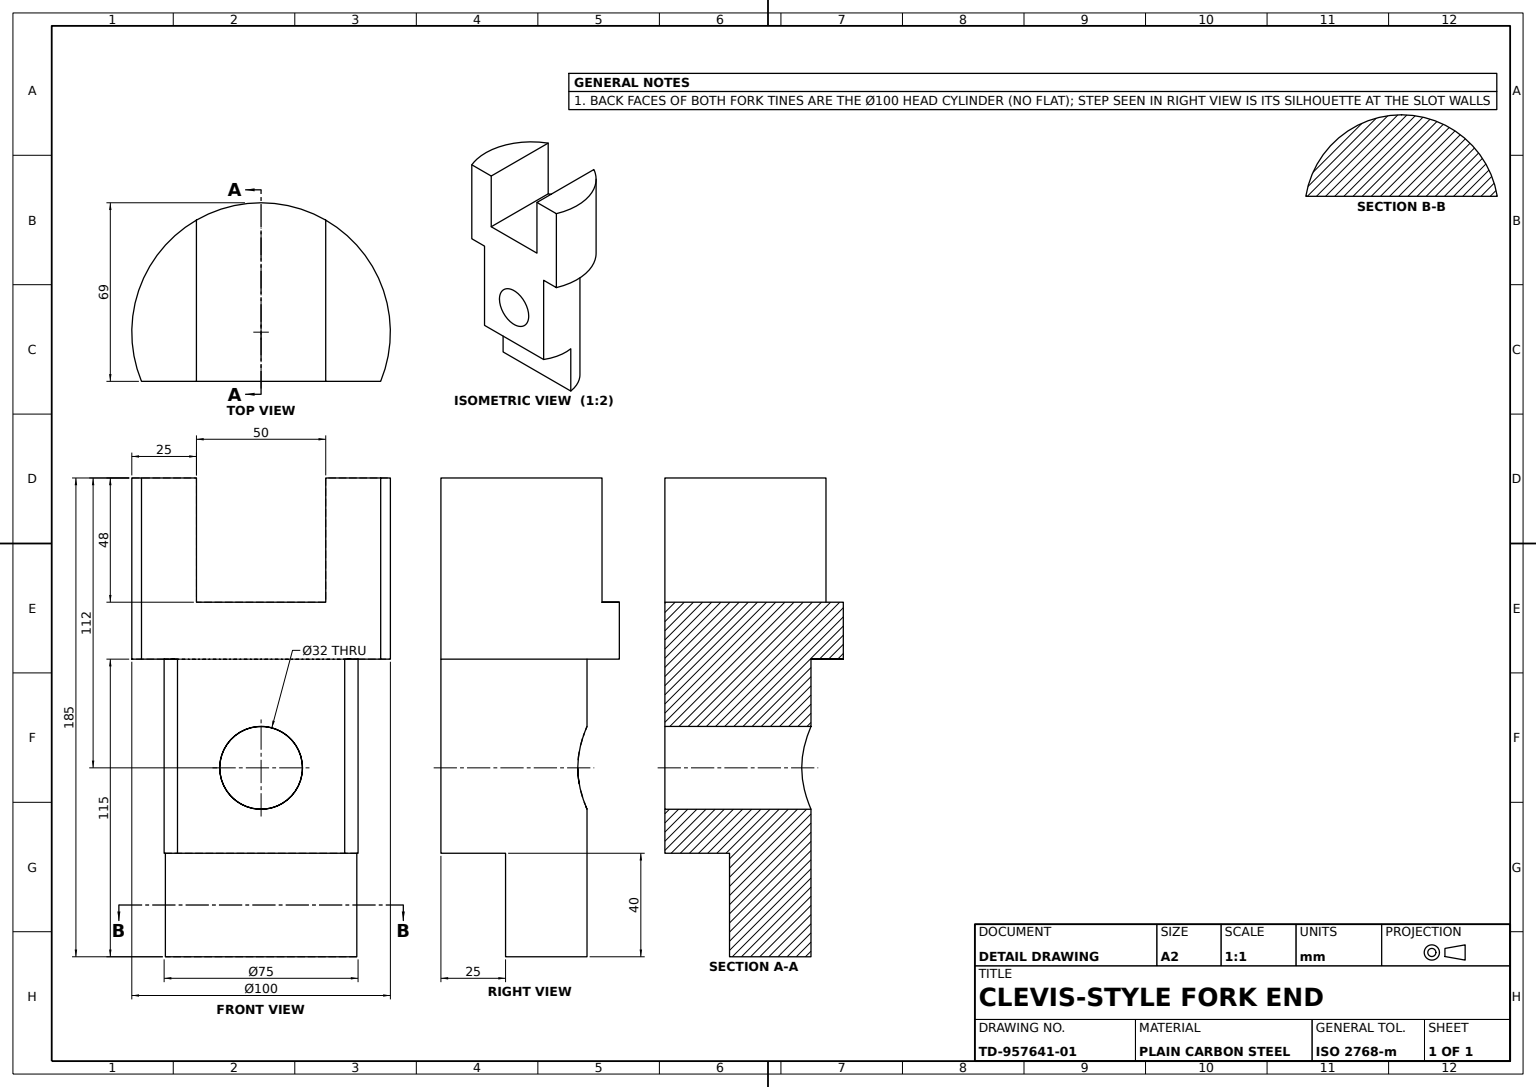
from build123d import *

# Parameters (mm, degrees)
SHANK_PROFILE_75_R   = 37.5
SHANK_75_DEPTH       = 115
HEAD_PROFILE_100_R   = 50
FORK_HEAD_100_DEPTH  = 70
FLAT_FACE_CUT_DEPTH  = 230
FORK_SLOT_PROFILE_R  = 16
FORK_SLOT_PROFILE_W  = 50
FORK_SLOT_PROFILE_H  = 62.840020357
FORK_SLOT_CUT_DEPTH  = 230
CROSS_HOLE_PROFILE_W = 75
CROSS_HOLE_PROFILE_H = 40
CROSS_HOLE_CUT_DEPTH = 25


with BuildPart() as part:
    # Shank Profile Ø75 → Shank Ø75 (new body)
    with BuildSketch(Plane(origin=(0, 0, 0), x_dir=(1, 0, 0), z_dir=(0, 1, 0))):
        with Locations(Location((0, 0, 0), (0, 0, 270))):
            Circle(SHANK_PROFILE_75_R)
    extrude(amount=SHANK_75_DEPTH)

    # Head Profile Ø100 → Fork Head Ø100 (add)
    with BuildSketch(Plane(origin=(0, 115, 0), x_dir=(1, 0, 0), z_dir=(0, 1, 0))):
        with Locations(Location((0, 0, 0), (0, 0, 270))):
            Circle(HEAD_PROFILE_100_R)
    extrude(amount=FORK_HEAD_100_DEPTH)

    # Flat Face Profile → Flat Face Cut (cut)
    with BuildSketch(Plane(origin=(0, 185, 0), x_dir=(1, 0, 0), z_dir=(0, 1, 0))):
        Polygon((-81.032063785, -19), (77.121249896, -19), (5.631572001, -69.155704166), align=None)
    extrude(amount=-FLAT_FACE_CUT_DEPTH, mode=Mode.SUBTRACT)

    # Fork Slot Profile → Fork Slot Cut (cut)
    with BuildSketch(Plane.XY.offset(19)):
        with Locations((0, 73)):
            Circle(FORK_SLOT_PROFILE_R)
        with Locations((0, 168.420010179)):
            Rectangle(FORK_SLOT_PROFILE_W, FORK_SLOT_PROFILE_H)
    extrude(amount=-FORK_SLOT_CUT_DEPTH, mode=Mode.SUBTRACT)

    # Cross Hole Profile → Cross Hole Cut (cut)
    with BuildSketch(Plane.XY.offset(19)):
        with Locations((0, 20)):
            Rectangle(CROSS_HOLE_PROFILE_W, CROSS_HOLE_PROFILE_H)
    extrude(amount=-CROSS_HOLE_CUT_DEPTH, mode=Mode.SUBTRACT)


solid = part.part
